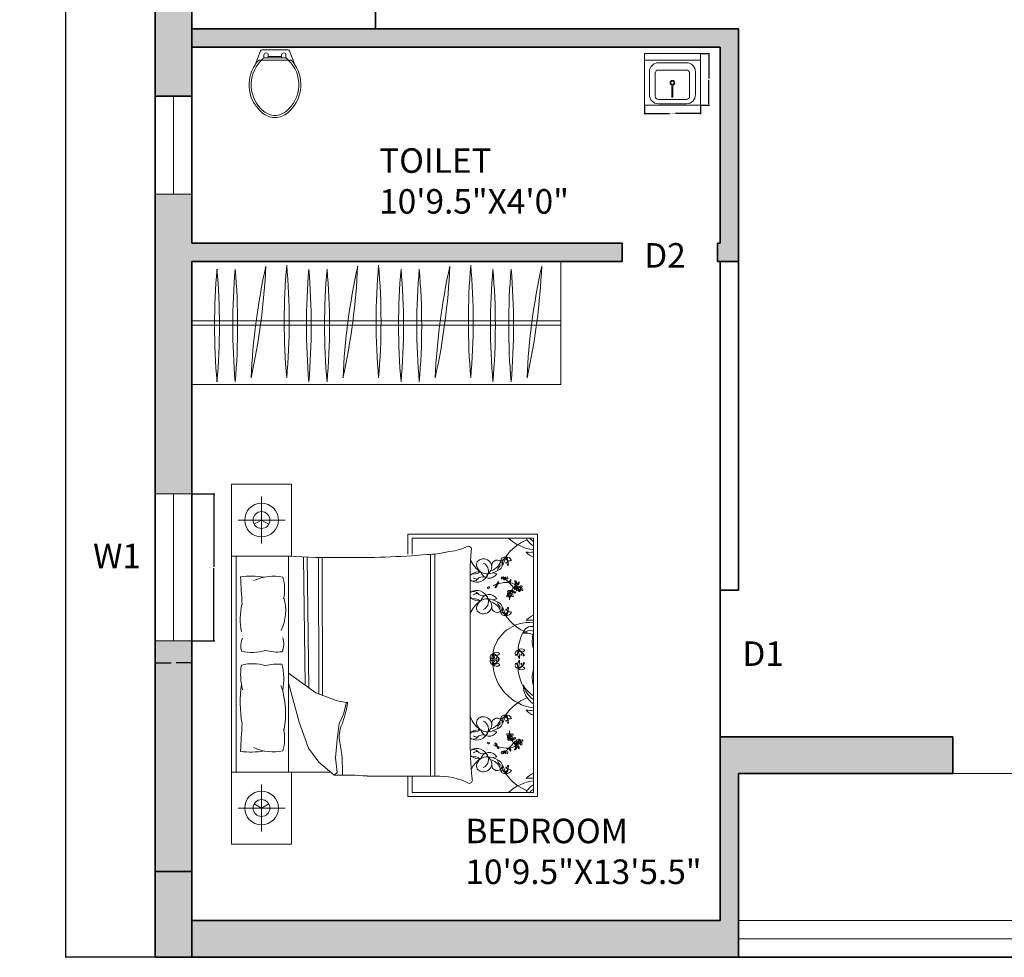
# Model space of a CAD drawing. Units: inches. Extents: x -9 to 505, y -680 to 48.
# Tile 1 of 17: x -6 to 235, y -680 to -450. Entities that reach past the tile are written whole.
import ezdxf

# ---------------------------------------------------------------- set-up
doc = ezdxf.new("R2010")
doc.units = ezdxf.units.IN
doc.header["$MEASUREMENT"] = 0
for name, color, linetype, lineweight in [('A-ANNO-DIMS', 2, 'Continuous', 18), ('A-ANNO-TEXT', 7, 'Continuous', 18), ('A-AREA-IDEN', 7, 'Continuous', 18), ('A-FLOR-CASE', 8, 'Continuous', 18), ('A-FLOR-FIXT', 9, 'Continuous', 18), ('A-FLOR-HRAL', 4, 'Continuous', 18), ('A-FURN', 8, 'Continuous', 18), ('A-GLAZ', 4, 'Continuous', 18), ('A-WALL', 7, 'Continuous', 35), ('A-WALL-PATT', 251, 'Continuous', 13), ('S-CONC', 7, 'Continuous', 35), ('S-CONC-PATT', 18, 'Continuous', 13), ('WC-Detail_dwgmodels.com', 251, 'Continuous', 13), ('WC-Outline_dwgmodels.com', 250, 'Continuous', 18)]:
    doc.layers.add(name, color=color, linetype=linetype, lineweight=lineweight)
doc.styles.get("Standard").update_dxf_attribs({"font": 'arial.ttf'})
doc.dimstyles.get("Standard").update_dxf_attribs({"dimtxt": 0.18, "dimasz": 0.18, "dimexe": 0.18, "dimexo": 0.0625, "dimgap": 0.09, "dimtad": 0, "dimtih": 1, "dimtoh": 1, "dimdec": 0, "dimzin": 0, "dimdsep": 46, "dimlunit": 3, "dimtxsty": 'Standard', "dimcen": 0.09, "dimadec": 0, "dimazin": 0, "dimtfac": 1, "dimtdec": 0, "dimtofl": 0, "dimtmove": 0, "dimatfit": 3, "dimfxl": 1, "dimtolj": 1, "dimtzin": 0, "dimarcsym": 0})

# ---------------------------------------------------------------- blocks, each defined once
blk = doc.blocks.new('*D3')
at = {"layer": 'A-ANNO-DIMS', "color": 0, "lineweight": -2, "transparency": 16777216}
for p, q in [((27.2, 11.5), (5.16, 11.5)), ((5.34, 11.32), (5.34, -330.86)), ((5.34, -679.32), (5.34, -337.14)), ((27.2, -679.5), (5.16, -679.5))]:
    blk.add_line(p, q, dxfattribs=at)
at = {"layer": 'A-ANNO-DIMS', "color": 0, "transparency": 16777216}
for points in [[(5.31, 11.32), (5.37, 11.32), (5.34, 11.5)], [(5.31, -679.32), (5.37, -679.32), (5.34, -679.5)]]:
    blk.add_solid(points, dxfattribs=at)
at = {"layer": 'Defpoints', "color": 0, "transparency": 16777216}
for p in [(27.26, 11.5), (5.34, -679.5), (27.26, -679.5)]:
    blk.add_point(p, dxfattribs=at)
at = {"layer": 'A-ANNO-DIMS', "color": 0, "transparency": 16777216, "insert": (5.34, -334), "char_height": 6, "attachment_point": 5}
blk.add_mtext('\\A1;57\'-7"', dxfattribs=at)
blk = doc.blocks.new('М14 600х655')
for p, q in [((-655, 600), (-655, 0)), ((-655, 600), (-655, 0)), ((-655, 0), (-655, 600)), ((0, 600), (-655, 600)), ((0, 0), (0, 600)), ((0, 525), (-655, 525)), ((-165, 494), (-490, 494)), ((-596, 388), (-596, 121)), ((-528, 370), (-528, 103)), ((-165, 408), (-490, 408)), ((-127, 103), (-127, 370)), ((-59, 121), (-59, 388)), ((-334, 87), (-334, 220)), ((-321, 87), (-321, 220)), ((-655, 0), (-655, 0)), ((-655, 0), (-655, 0)), ((-655, 0), (0, 0)), ((-655, 0), (0, 0)), ((-490, 65), (-165, 65)), ((-490, 15), (-165, 15))]:
    blk.add_line(p, q)
for radius in [27.6, 19.3]:
    blk.add_circle((-327, 259), radius)
for centre, radius, start, end in [((-490, 388), 106, 90, 180), ((-165, 388), 106, 0, 90), ((-490, 370), 38.2, 90, 180), ((-165, 370), 38.2, 0, 90), ((-490, 121), 106, 180, 270), ((-165, 121), 106, 270, 0), ((-490, 103), 38.2, 180, 270), ((-165, 103), 38.2, 270, 0)]:
    blk.add_arc(centre, radius, start, end)
blk = doc.blocks.new('WIN-36')
for p, q in [((0, 36), (0, 0)), ((9, 36), (0, 36)), ((4.5, 36), (4.5, 2.23)), ((9, 0), (9, 36)), ((0, 0), (9, 0)), ((4.5, 2.23), (4.5, 0))]:
    blk.add_line(p, q)
blk = doc.blocks.new('WIN-24')
for p, q in [((0, 24), (0, 0)), ((9, 24), (0, 24)), ((4.5, 24), (4.5, 2.23)), ((9, 0), (9, 24)), ((0, 0), (9, 0)), ((4.5, 2.23), (4.5, 0))]:
    blk.add_line(p, q)
blk = doc.blocks.new('*D16')
at = {"layer": 'A-ANNO-DIMS', "color": 0, "lineweight": -2, "transparency": 16777216}
for p, q in [((36.33, -565.96), (41.84, -565.96)), ((41.66, -566.14), (41.66, -583.78)), ((41.66, -601.78), (41.66, -584.14)), ((36.33, -601.96), (41.84, -601.96))]:
    blk.add_line(p, q, dxfattribs=at)
at = {"layer": 'A-ANNO-DIMS', "color": 0, "transparency": 16777216}
for points in [[(41.63, -566.14), (41.69, -566.14), (41.66, -565.96)], [(41.63, -601.78), (41.69, -601.78), (41.66, -601.96)]]:
    blk.add_solid(points, dxfattribs=at)
at = {"layer": 'Defpoints', "color": 0, "transparency": 16777216}
for p in [(36.26, -565.96), (41.66, -565.96), (36.26, -601.96)]:
    blk.add_point(p, dxfattribs=at)
at = {"layer": 'A-ANNO-DIMS', "color": 0, "transparency": 16777216, "insert": (41.66, -583.96), "char_height": 0.18, "attachment_point": 5}
blk.add_mtext('\\A1;WINDOW 3\'-0" TYP.', dxfattribs=at)
blk = doc.blocks.new('*D17')
at = {"layer": 'A-ANNO-DIMS', "color": 0, "lineweight": -2, "transparency": 16777216}
for p, q in [((27.26, -602.02), (27.26, -607.54)), ((36.26, -602.02), (36.26, -607.54)), ((27.44, -607.36), (31.12, -607.36)), ((36.08, -607.36), (32.4, -607.36))]:
    blk.add_line(p, q, dxfattribs=at)
at = {"layer": 'A-ANNO-DIMS', "color": 0, "transparency": 16777216}
for points in [[(27.44, -607.33), (27.44, -607.39), (27.26, -607.36)], [(36.08, -607.33), (36.08, -607.39), (36.26, -607.36)]]:
    blk.add_solid(points, dxfattribs=at)
at = {"layer": 'Defpoints', "color": 0, "transparency": 16777216}
for p in [(27.26, -601.96), (36.26, -601.96), (36.26, -607.36)]:
    blk.add_point(p, dxfattribs=at)
at = {"layer": 'A-ANNO-DIMS', "color": 0, "transparency": 16777216, "insert": (31.76, -607.36), "char_height": 0.18, "attachment_point": 5}
blk.add_mtext('\\A1;0\'-9" TYP.', dxfattribs=at)
blk = doc.blocks.new('*D30')
at = {"layer": 'A-ANNO-DIMS', "color": 0, "lineweight": -2, "transparency": 16777216}
for p, q in [((147.17, -470.73), (147.17, -472.91)), ((147.35, -472.73), (153.31, -472.73)), ((160.75, -472.73), (154.79, -472.73)), ((160.93, -470.73), (160.93, -472.91))]:
    blk.add_line(p, q, dxfattribs=at)
at = {"layer": 'A-ANNO-DIMS', "color": 0, "transparency": 16777216}
for points in [[(147.35, -472.7), (147.35, -472.76), (147.17, -472.73)], [(160.75, -472.7), (160.75, -472.76), (160.93, -472.73)]]:
    blk.add_solid(points, dxfattribs=at)
at = {"layer": 'Defpoints', "color": 0, "transparency": 16777216}
for p in [(147.17, -470.66), (160.93, -470.66), (160.93, -472.73)]:
    blk.add_point(p, dxfattribs=at)
at = {"layer": 'A-ANNO-DIMS', "color": 0, "transparency": 16777216, "insert": (154.05, -472.73), "char_height": 0.18, "attachment_point": 5}
blk.add_mtext('\\A1;BASIN 1\'-2"', dxfattribs=at)
blk = doc.blocks.new('*D31')
at = {"layer": 'A-ANNO-DIMS', "color": 0, "lineweight": -2, "transparency": 16777216}
for p, q in [((160.99, -458.06), (163.18, -458.06)), ((163, -458.24), (163, -464.18)), ((163, -470.48), (163, -464.54)), ((160.99, -470.66), (163.18, -470.66))]:
    blk.add_line(p, q, dxfattribs=at)
at = {"layer": 'A-ANNO-DIMS', "color": 0, "transparency": 16777216}
for points in [[(162.97, -458.24), (163.03, -458.24), (163, -458.06)], [(162.97, -470.48), (163.03, -470.48), (163, -470.66)]]:
    blk.add_solid(points, dxfattribs=at)
at = {"layer": 'Defpoints', "color": 0, "transparency": 16777216}
for p in [(160.93, -458.06), (163, -458.06), (160.93, -470.66)]:
    blk.add_point(p, dxfattribs=at)
at = {"layer": 'A-ANNO-DIMS', "color": 0, "transparency": 16777216, "insert": (163, -464.36), "char_height": 0.18, "attachment_point": 5}
blk.add_mtext('\\A1;1\'-0 1/2"', dxfattribs=at)

msp = doc.modelspace()

# ---------------------------------------------------------------- hatches: boundary and pattern name
at = {"layer": 'A-WALL-PATT'}
h = msp.add_hatch(color=256, dxfattribs=at)
h.dxf.hatch_style = 1
h.paths.add_polyline_path([(101.64, 11.5), (48.26, 11.5), (48.26, 2.5), (72.26, 2.5), (72.26, -21.25), (81.26, -21.25), (81.26, 2.5), (101.64, 2.5)])
h.paths.add_polyline_path([(36.26, 2.5), (27.26, 2.5), (27.26, -6.92), (36.26, -6.92)])
h.paths.add_polyline_path([(81.26, -57.25), (72.26, -57.25), (72.26, -75.5), (81.26, -75.5)])
h.paths.add_polyline_path([(162.76, 11.5), (137.64, 11.5), (137.64, 2.5), (162.76, 2.5)])
h.paths.add_polyline_path([(179.26, 2.5), (174.76, 2.5), (174.76, -75.5), (179.26, -75.5), (179.26, -54.5), (229.51, -54.5), (229.51, -45.5), (179.26, -45.5)])
h.paths.add_polyline_path([(382.26, -45.5), (332.26, -45.5), (332.26, 2.5), (327.76, 2.5), (327.76, -45.5), (277.51, -45.5), (277.51, -54.5), (327.76, -54.5), (327.76, -111.5), (332.26, -111.5), (332.26, -54.5), (382.26, -54.5)])
h.paths.add_polyline_path([(332.26, -128), (327.76, -128), (327.76, -207), (332.26, -207)])
h.paths.add_polyline_path([(124.76, -111.5), (36.26, -111.5), (36.26, -116), (120.26, -116), (120.26, -168.5), (179.26, -168.5), (179.26, -164), (124.76, -164)])
h.paths.add_polyline_path([(96.26, -164), (36.26, -164), (36.26, -152), (27.26, -152), (27.26, -208.88), (36.26, -208.88), (36.26, -168.5), (96.26, -168.5)])
h.paths.add_polyline_path([(36.26, -244.88), (27.26, -244.88), (27.26, -287), (36.26, -287)])
h.paths.add_polyline_path([(179.26, -204.5), (174.76, -204.5), (174.76, -287), (179.26, -287)])
h.paths.add_polyline_path([(257.26, -296), (248.26, -296), (248.26, -446), (269.26, -446), (269.26, -437), (257.26, -437)])
h.paths.add_polyline_path([(90.26, -296), (81.26, -296), (81.26, -348.67), (90.26, -348.67)])
h.paths.add_polyline_path([(90.26, -384.67), (81.26, -384.67), (81.26, -416), (90.26, -416)])
h.paths.add_polyline_path([(170.26, -452), (36.26, -452), (36.26, -456.5), (165.76, -456.5), (165.76, -504.5), (165.13, -504.5), (165.13, -509), (170.26, -509)])
h.paths.add_polyline_path([(141.76, -504.5), (36.26, -504.5), (36.26, -492.5), (27.26, -492.5), (27.26, -565.96), (36.26, -565.96), (36.26, -509), (141.76, -509)])
h.paths.add_polyline_path([(36.26, -601.96), (27.26, -601.96), (27.26, -658.5), (36.26, -658.5)])
h.paths.add_polyline_path([(170.26, -670.5), (170.26, -634.5), (222.76, -634.5), (222.76, -625.5), (165.76, -625.5), (165.76, -670.5), (36.26, -670.5), (36.26, -679.5), (170.26, -679.5)])
h.paths.add_polyline_path([(332.26, -616.5), (433.89, -616.5), (433.89, -612), (332.26, -612), (332.26, -610.56), (327.76, -610.56), (327.76, -625.5), (270.76, -625.5), (270.76, -634.5), (327.76, -634.5), (327.76, -658.5), (332.26, -658.5)])
h.paths.add_polyline_path([(459.76, -670.5), (336.76, -670.5), (336.76, -679.5), (459.76, -679.5)])
h.paths.add_polyline_path([(468.76, -545.74), (459.76, -545.74), (459.76, -612), (457.89, -612), (457.89, -616.5), (459.76, -616.5), (459.76, -658.5), (468.76, -658.5)])
h.paths.add_polyline_path([(332.26, -446), (327.76, -446), (327.76, -574.56), (332.26, -574.56)])
h.paths.add_polyline_path([(327.76, -437), (305.26, -437), (305.26, -446), (327.76, -446)])
h.paths.add_polyline_path([(459.76, -437), (348.76, -437), (348.76, -446), (459.76, -446)])
h.paths.add_polyline_path([(468.76, -458), (459.76, -458), (459.76, -509.74), (468.76, -509.74)])
h.paths.add_polyline_path([(468.76, -365), (459.76, -365), (459.76, -437), (468.76, -437)])
h.paths.add_polyline_path([(468.76, -299.6), (459.76, -299.6), (459.76, -344), (468.76, -344)])
h.paths.add_polyline_path([(468.76, -184.74), (459.76, -184.74), (459.76, -231), (401.26, -231), (401.26, -235.5), (459.76, -235.5), (459.76, -275.6), (468.76, -275.6)])
h.paths.add_polyline_path([(390.76, -356), (342.76, -356), (342.76, -365), (390.76, -365)])
h.paths.add_polyline_path([(459.76, -356), (405.76, -356), (405.76, -365), (459.76, -365)])
h.paths.add_polyline_path([(405.76, -296), (396.76, -296), (396.76, -356), (405.76, -356)])
h.paths.add_polyline_path([(336.76, -296), (327.76, -296), (327.76, -356), (336.76, -356)])
h.paths.add_polyline_path([(468.76, -9.5), (459.76, -9.5), (459.76, -45.5), (418.26, -45.5), (418.26, -54.5), (468.76, -54.5)])
h.paths.add_polyline_path([(468.76, -54.5), (459.76, -54.5), (459.76, -111.5), (468.76, -111.5)])
h.paths.add_polyline_path([(468.76, -128), (459.76, -128), (459.76, -148.74), (468.76, -148.74)])
at = {"layer": 'S-CONC-PATT'}
h = msp.add_hatch(color=256, dxfattribs=at)
h.dxf.hatch_style = 1
h.paths.add_polyline_path([(36.26, -447.5), (27.26, -447.5), (27.26, -468.5), (36.26, -468.5), (36.26, -456.5), (36.26, -452)])
h = msp.add_hatch(color=256, dxfattribs=at)
h.dxf.hatch_style = 1
h.paths.add_polyline_path([(336.76, -658.5), (327.76, -658.5), (327.76, -679.5), (336.76, -679.5), (336.76, -670.5)])
h.paths.add_polyline_path([(468.76, -658.5), (459.76, -658.5), (459.76, -679.5), (468.76, -679.5)])
h.paths.add_polyline_path([(36.26, -658.5), (27.26, -658.5), (27.26, -679.5), (36.26, -679.5)])

# ---------------------------------------------------------------- linework, layer by layer
at = {"layer": 'A-FLOR-CASE'}
for p, q in [((126.66, -509), (36.26, -509)), ((36.26, -509), (36.26, -539.13)), ((126.66, -509), (126.66, -539.13)), ((126.66, -523.56), (36.26, -523.56)), ((126.66, -524.57), (36.26, -524.57)), ((126.66, -539.13), (36.26, -539.13))]:
    msp.add_line(p, q, dxfattribs=at)
for centre, start, end in [((200.34, -524.67), 175.0028, 184.9972), ((-115.55, -524.67), 355.0028, 4.9972), ((204.8, -524.67), 175.0028, 184.9972), ((-111.08, -524.67), 355.0028, 4.9972), ((-104.03, -503.22), 347.508, 357.5023), ((209.16, -544.42), 167.508, 177.5023), ((217.43, -523.7), 175.0028, 184.9972), ((-98.45, -523.7), 355.0028, 4.9972), ((222.86, -524.67), 175.0028, 184.9972), ((-93.03, -524.67), 355.0028, 4.9972), ((227.32, -524.67), 175.0028, 184.9972), ((-88.56, -524.67), 355.0028, 4.9972), ((-81.51, -503.22), 347.508, 357.5023), ((231.68, -544.42), 167.508, 177.5023), ((239.95, -523.7), 175.0028, 184.9972), ((-75.93, -523.7), 355.0028, 4.9972), ((245.46, -524.67), 175.0028, 184.9972), ((-70.42, -524.67), 355.0028, 4.9972), ((249.93, -524.67), 175.0028, 184.9972), ((-65.96, -524.67), 355.0028, 4.9972), ((254.28, -544.42), 167.508, 177.5023), ((-58.9, -503.22), 347.508, 357.5023), ((262.56, -523.7), 175.0028, 184.9972), ((-53.33, -523.7), 355.0028, 4.9972), ((267.98, -524.67), 175.0028, 184.9972), ((-47.9, -524.67), 355.0028, 4.9972), ((272.45, -524.67), 175.0028, 184.9972), ((-43.43, -524.67), 355.0028, 4.9972), ((276.8, -544.42), 167.508, 177.5023), ((-36.38, -503.22), 347.508, 357.5023)]:
    msp.add_arc(centre, 158.54, start, end, dxfattribs=at)
at = {"layer": 'A-FLOR-HRAL'}
for p, q in [((170.26, -670.5), (170.26, -679.5)), ((327.76, -670.5), (170.26, -670.5)), ((170.26, -670.5), (327.76, -670.5)), ((170.26, -675), (327.76, -675)), ((170.26, -679.5), (327.76, -679.5))]:
    msp.add_line(p, q, dxfattribs=at)
at = {"layer": 'A-FURN'}
for p, q in [((45.97, -651.75), (45.97, -563.54)), ((53.32, -578.12), (53.32, -566.59)), ((59.09, -572.36), (47.56, -572.36)), ((89.21, -580.69), (89.21, -575.8)), ((89.21, -575.8), (120.99, -575.8)), ((90.23, -576.82), (90.23, -580.71)), ((119.97, -576.82), (90.23, -576.82)), ((119.97, -639.08), (119.97, -576.82)), ((120.99, -575.8), (120.99, -640.1)), ((47.1, -581.18), (47.1, -634.11)), ((59.91, -634.11), (59.91, -581.18)), ((63.58, -581.42), (64.02, -612.82)), ((64.48, -581.45), (64.93, -613.48)), ((67.26, -581.5), (67.39, -614.99)), ((68.16, -581.49), (68.3, -615.34)), ((94.71, -580.78), (94.71, -635.12)), ((95.81, -580.69), (95.81, -635.12)), ((111.02, -585.51), (110.03, -585.32)), ((104.48, -589.73), (104.48, -625.55)), ((111.02, -591.67), (110.03, -591.87)), ((59.91, -609.87), (66.64, -614.71)), ((62.53, -621.85), (59.91, -612.23)), ((66.64, -614.71), (71.82, -616.67)), ((71.82, -616.67), (74.14, -617.03)), ((74.14, -617.03), (73.42, -619.89)), ((73.42, -619.89), (72.35, -622.21)), ((64.85, -628.28), (62.53, -621.85)), ((72.35, -622.21), (71.82, -626.14)), ((111.02, -624.22), (110.03, -624.03)), ((71.82, -626.14), (71.46, -630.61)), ((67.35, -631.68), (64.85, -628.28)), ((71.1, -634.89), (67.35, -631.68)), ((71.46, -630.61), (71.82, -634.18)), ((111.02, -630.39), (110.03, -630.58)), ((45.97, -634.11), (70.18, -634.11)), ((71.82, -634.18), (71.1, -634.89)), ((53.32, -637.16), (53.32, -648.69)), ((89.21, -640.1), (89.21, -635.11)), ((90.23, -635.12), (90.23, -639.08)), ((90.23, -639.08), (119.97, -639.08)), ((120.99, -640.1), (89.21, -640.1)), ((59.09, -642.93), (47.56, -642.93))]:
    msp.add_line(p, q, dxfattribs=at)
for points in [[(45.97, -581.18), (60.67, -581.18), (60.67, -563.54), (45.97, -563.54)], [(53.32, -572.36), (51.54, -573.39)], [(53.32, -572.36), (55.1, -573.39)], [(60.67, -634.11), (60.67, -651.75), (45.97, -651.75)], [(53.32, -642.93), (51.54, -641.9)], [(53.32, -642.93), (55.1, -641.9)]]:
    msp.add_lwpolyline(points, dxfattribs=at)
for points in [[(94.02, -580.8, 0.056112), (98.87, -580.16, 0.095341), (103.55, -578.92)], [(48.17, -586.25, -0.074897), (53.93, -586.35, 0.472817)], [(54.25, -604.29, -0.14099), (48.38, -604.46, -0.235245)], [(54.25, -608.06, 0.14099), (48.38, -607.88, 0.235245)], [(48.17, -629.04, 0.074897), (53.93, -628.93, -0.472817)], [(79.18, -635.08, 0.001242), (95.92, -635.12, -0.127202), (104.26, -636.89)]]:
    msp.add_lwpolyline(points, format="xyb", dxfattribs=at)
for centre, radius in [((53.32, -572.36), 4.12), ((53.32, -572.36), 2.06), ((116.59, -589.14), 0.225), ((114.22, -590.61), 0.225), ((114.22, -625.29), 0.225), ((116.59, -626.76), 0.225), ((53.32, -642.93), 4.12), ((53.32, -642.93), 2.06)]:
    msp.add_circle(centre, radius, dxfattribs=at)
for centre, radius, start, end in [((121.52, -568.24), 11.52, 228.1144, 262.255), ((123.06, -574.02), 5.61, 209.8884, 236.5383), ((124.11, -572), 6.99, 223.5186, 233.6964), ((104, -579.59), 0.804, 336.5219, 123.8264), ((122.66, -587.95), 11.52, 111.4092, 145.6135), ((70.69, -423.05), 158.5, 266.1, 270.9282), ((76.45, -374.79), 206.76, 269.1145, 274.8735), ((190.27, -587.03), 85.84, 175.2402, 181.8035), ((112.92, -582.37), 0.955, 76.272, 177.0484), ((111.47, -580.42), 1.97, 284.7031, 328.6173), ((114.22, -582.92), 1.82, 125.7657, 194.5347), ((105.28, -579.7), 8.06, 332.8176, 347.4827), ((113.42, -582.69), 1.28, 20.9613, 102.2885), ((114.11, -581.41), 0.962, 181.7131, 301.5367), ((110.96, -583.36), 2.91, 2.0648, 41.1598), ((112.71, -582.28), 0.942, 316.2238, 62.3173), ((121.76, -577.16), 4.68, 221.0454, 247.4453), ((119.25, -564.33), 15.94, 266.3481, 272.5919), ((110.69, -579.48), 6.68, 203.6453, 236.3329), ((107.49, -583.37), 1.49, 88.9462, 185.5144), ((108.59, -582.91), 2.65, 193.079, 274.7067), ((107.7, -583.98), 2.11, 7.1143, 95.0551), ((106.9, -584.81), 2.05, 338.5779, 68.4181), ((107.23, -583.61), 2.56, 305.9599, 357.6409), ((108.18, -580.87), 4.16, 288.2955, 328.7386), ((111.09, -583.49), 1.32, 19.1312, 189.736), ((110.7, -583.17), 1.65, 285.6955, 4.031), ((112.89, -584.96), 1.76, 128.4175, 173.8338), ((112.53, -583.22), 0.811, 126.7319, 206.0245), ((113.26, -582.83), 0.0751, 20.2667, 316.2271), ((113.73, -583.26), 0.143, 168.5166, 2.0648), ((113.65, -583.25), 0.0695, 52.0591, 168.5166), ((-791.3, -634.87), 840.88, 2.85022, 3.31479), ((56.24, -597.48), 11.37, 78.2417, 114.8684), ((47.14, -589.39), 11.82, 348.9631, 14.8961), ((105.45, -586.45), 1.06, 127.675, 162.5814), ((105.13, -581.93), 3.65, 259.249, 301.1782), ((106.08, -584.76), 2.81, 240.8249, 340.7178), ((106.72, -588.43), 3.4, 85.2696, 124.215), ((106.59, -584.33), 2.54, 240.0851, 262.564), ((107.58, -588.08), 1.81, 74.8529, 138.4347), ((109.12, -584.42), 2.19, 196.8663, 330.0915), ((108.2, -585.81), 0.547, 254.8529, 12.6959), ((106.72, -588.43), 3.4, 53.6555, 57.2989), ((108.52, -580.83), 4.73, 273.4924, 303.7117), ((112.27, -586.63), 0.174, 125.0752, 284.7644), ((112.54, -586.56), 0.375, 127.3642, 168.4363), ((112.24, -586.26), 0.54, 277.4968, 341.2737), ((112.67, -586.51), 0.215, 88.1325, 178.8919), ((113.1, -586.74), 0.464, 136.3462, 189.6513), ((112.88, -586.25), 0.225, 183.2768, 356.7232), ((113.59, -586.65), 0.735, 164.2829, 186.9148), ((112.72, -586.66), 0.368, 312.3208, 40.2111), ((113.5, -586.24), 0.522, 201.6382, 274.947), ((112.81, -586.96), 0.682, 42.3896, 66.5724), ((113.3, -586.56), 0.371, 10.9597, 52.2379), ((113.53, -586.59), 0.172, 274.947, 37.5263), ((105.45, -586.45), 1.06, 196.6343, 225.5483), ((105.24, -586), 1.32, 246.1646, 318.4347), ((108.93, -588.83), 0.276, 169.5864, 349.5616), ((109.03, -588.85), 0.17, 349.5616, 167.2949), ((113.47, -594.96), 7.31, 110.1059, 116.9968), ((111.02, -588.94), 0.463, 129.5056, 182.6421), ((109.69, -587.87), 1.39, 308.4388, 328.836), ((109.45, -586.73), 2.49, 296.5064, 305.3102), ((109.43, -588.01), 1.42, 336.3901, 344.4871), ((110.97, -588.37), 0.18, 83.9457, 185.6216), ((110.25, -588.21), 0.739, 328.836, 0.8141), ((110.63, -588.42), 0.423, 306.5232, 32.4668), ((111.14, -588.09), 0.18, 112.5583, 214.2343), ((111.02, -587.77), 0.423, 265.7131, 351.6568), ((110.65, -587.54), 0.739, 297.3659, 329.344), ((110.09, -586.9), 1.42, 313.6929, 321.7899), ((111.66, -587.87), 0.463, 115.5379, 168.6744), ((110.09, -587.21), 1.39, 329.344, 349.7412), ((113.47, -594.96), 7.31, 86.1723, 106.4158), ((108.97, -587.53), 2.49, 352.8698, 1.6736), ((112.84, -586.79), 0.194, 189.6513, 312.3208), ((119.69, -581.56), 8.38, 217.9541, 226.8459), ((114.11, -587.57), 0.18, 112.5583, 214.2343), ((113.99, -587.25), 0.423, 265.7131, 351.6568), ((113.62, -587.01), 0.739, 297.3659, 329.344), ((113.66, -591.32), 3.66, 60.7959, 85.244), ((105.86, -596.59), 12.05, 37.8256, 47.7588), ((113.06, -586.38), 1.42, 313.6929, 321.7899), ((114.63, -587.35), 0.463, 115.5379, 168.6744), ((113.06, -586.68), 1.39, 329.344, 349.7412), ((111.94, -587), 2.49, 352.8698, 1.6736), ((118.52, -591.7), 4.39, 130.182, 149.456), ((115.44, -587.5), 0.251, 33.0979, 123.1364), ((109.91, -591.04), 6.56, 31.1156, 34.8118), ((115.08, -587.93), 0.679, 2.3172, 70.5201), ((116.1, -589.19), 0.724, 139.3812, 199.9959), ((114.75, -588.67), 1.02, 310.9365, 22.7695), ((115.64, -588.1), 0.196, 135.7354, 318.1297), ((115.31, -587.78), 0.26, 315.7354, 31.1156), ((115.09, -588.33), 0.603, 319.3812, 5.5456), ((115.78, -588.1), 0.196, 68.2452, 250.6395), ((115.33, -587.86), 0.585, 352.6008, 57.1845), ((117.42, -591.78), 3.91, 111.7087, 116.2181), ((113.66, -591.32), 3.66, 47.5083, 55.9967), ((115.89, -587.72), 0.585, 252.8042, 349.6943), ((115.33, -588.77), 0.622, 331.1838, 51.6792), ((115.95, -587.68), 0.26, 248.2452, 323.6254), ((115.72, -587.52), 0.679, 291.7087, 3.0299), ((116.19, -588.85), 0.22, 138.2946, 276.2474), ((116.28, -588.89), 0.306, 358.5719, 143.8954), ((110.88, -583.94), 6.56, 323.6254, 327.3216), ((116.45, -588.65), 0.309, 208.8493, 269.9355), ((116.19, -588.72), 0.353, 274.2123, 318.1587), ((116.26, -587.69), 0.251, 325.6077, 55.6462), ((117.27, -589.08), 0.708, 121.9501, 165.2442), ((116.78, -588.8), 0.149, 262.868, 7.094), ((116.76, -588.68), 0.443, 278.5614, 22.5914), ((117.01, -588.66), 0.223, 44.3732, 121.9501), ((48.01, -594.49), 11.23, 333.8761, 16.1746), ((105.45, -590.73), 1.06, 134.4517, 156.7144), ((105.45, -590.73), 1.06, 203.2856, 232.325), ((106.08, -592.43), 2.81, 19.2822, 119.1751), ((105.24, -591.18), 1.32, 41.5653, 113.8354), ((106.59, -592.85), 2.54, 97.436, 119.9149), ((107.58, -589.11), 1.81, 221.5653, 285.1471), ((109.12, -592.77), 2.19, 29.9085, 163.1337), ((108.2, -591.38), 0.547, 347.3041, 105.1471), ((113.6, -590.98), 0.174, 125.0752, 284.7644), ((113.87, -590.92), 0.375, 93.635, 168.4363), ((113.89, -588.89), 1.02, 253.6301, 325.4631), ((114.17, -590.31), 0.724, 82.0748, 142.6895), ((114.09, -589.31), 0.744, 228.342, 274.9894), ((113.82, -590.32), 0.22, 138.2946, 276.2474), ((113.58, -590.62), 0.54, 277.4968, 341.2737), ((113.91, -590.36), 0.306, 358.5719, 143.8954), ((114.01, -590.87), 0.215, 88.1325, 178.8919), ((114.09, -590.12), 0.309, 208.8493, 269.9355), ((113.82, -590.19), 0.353, 274.2123, 318.1587), ((114.44, -591.1), 0.464, 136.3462, 189.6513), ((114.17, -591.14), 0.194, 189.6513, 312.3208), ((118.52, -591.7), 4.39, 175.2415, 182.8929), ((114.11, -589.43), 0.622, 273.8774, 357.1501), ((114.92, -591.01), 0.735, 164.2829, 186.9148), ((114.9, -590.55), 0.708, 121.9501, 165.2442), ((114.36, -588.99), 0.603, 262.0748, 308.2393), ((114.05, -591.01), 0.368, 312.3208, 40.2111), ((114.83, -590.6), 0.522, 201.6382, 274.947), ((114.41, -590.27), 0.149, 262.868, 7.094), ((114.14, -591.31), 0.682, 42.3896, 66.5724), ((114.39, -590.15), 0.443, 278.5614, 22.5914), ((114.64, -590.91), 0.371, 10.9597, 118.7804), ((118.52, -591.7), 4.39, 156.1523, 156.9499), ((114.64, -590.13), 0.223, 44.3732, 121.9501), ((115.33, -589.61), 0.622, 181.4625, 249.4747), ((115.22, -589.12), 0.603, 215.1128, 261.2773), ((115.7, -589.15), 1.02, 197.889, 269.722), ((114.86, -590.95), 0.172, 274.947, 37.5263), ((115.38, -589.5), 0.744, 248.3627, 295.0101), ((115.02, -590.43), 0.724, 20.6625, 81.2773), ((115.22, -588.73), 0.744, 285.6484, 332.2957), ((115.97, -589.51), 0.174, 125.0752, 284.7644), ((116.24, -589.45), 0.375, 93.635, 168.4363), ((115.95, -589.15), 0.54, 277.4968, 341.2737), ((116.38, -589.4), 0.215, 88.1325, 178.8919), ((116.81, -589.63), 0.464, 136.3462, 189.6513), ((116.54, -589.67), 0.194, 189.6513, 312.3208), ((117.29, -589.54), 0.735, 164.2829, 186.9148), ((116.42, -589.54), 0.368, 312.3208, 40.2111), ((117.2, -589.13), 0.522, 201.6382, 274.947), ((116.51, -589.84), 0.682, 42.3896, 66.5724), ((117, -589.44), 0.371, 10.9597, 118.7804), ((117.23, -589.48), 0.172, 274.947, 37.5263), ((63.6, -596.71), 15.51, 166.3427, 191.1841), ((105.13, -595.26), 3.65, 58.8218, 100.2867), ((110.69, -597.71), 6.68, 123.6671, 158.5059), ((106.72, -588.76), 3.4, 235.785, 274.7304), ((108.59, -594.28), 2.65, 85.2933, 166.921), ((107.49, -593.82), 1.49, 174.4856, 271.0538), ((107.7, -593.21), 2.11, 264.9449, 352.8857), ((106.9, -592.38), 2.05, 291.5819, 21.4221), ((106.72, -588.76), 3.4, 302.7011, 306.3445), ((107.23, -593.57), 2.56, 2.3591, 54.0401), ((108.52, -596.36), 4.73, 56.2883, 86.5076), ((108.18, -596.32), 4.16, 31.2614, 71.7045), ((111.09, -593.69), 1.32, 170.264, 340.8688), ((112.89, -592.23), 1.76, 186.1662, 231.5825), ((110.7, -594.01), 1.65, 355.969, 74.3045), ((112.53, -593.97), 0.811, 153.9755, 233.2681), ((114.22, -594.26), 1.82, 165.4653, 234.2343), ((105.28, -597.49), 8.06, 12.5173, 27.1824), ((113.73, -593.92), 0.143, 357.9352, 191.4834), ((112.92, -594.81), 0.955, 182.9516, 283.728), ((111.47, -596.77), 1.97, 31.3827, 75.2969), ((110.96, -593.82), 2.91, 318.8402, 357.9352), ((112.71, -594.91), 0.942, 297.6827, 43.7762), ((114.11, -595.77), 0.962, 58.4633, 178.2869), ((113.42, -594.49), 1.28, 257.7115, 339.0387), ((122.66, -589.24), 11.52, 214.3865, 248.5908), ((113.3, -594.34), 0.125, 43.7762, 339.7183), ((113.65, -593.94), 0.0695, 191.4834, 307.9409), ((121.76, -600.02), 4.68, 112.5547, 138.9546), ((118.86, -606.38), 8.91, 82.8636, 171.8197), ((119.48, -600.49), 2.07, 76.3898, 169.0739), ((119.25, -612.85), 15.94, 87.4081, 93.6519), ((127.69, -605.12), 11.52, 152.5854, 175.5377), ((119.2, -602.05), 2.61, 72.8609, 131.9049), ((118.04, -605.22), 5.16, 68.117, 96.6195), ((126.02, -601.9), 6.33, 162.9798, 196.4569), ((52.57, -603.25), 4.36, 153.3437, 196.1026), ((54.09, -602.66), 4.68, 335.0183, 18.5407), ((57.2, -593.89), 10.81, 254.1707, 275.9871), ((110.3, -606.02), 0.955, 106.1963, 206.9726), ((108.07, -605.06), 1.97, 314.6273, 358.5415), ((111.69, -605.86), 1.82, 155.6899, 224.4589), ((111.69, -607.1), 1.82, 135.5411, 204.3101), ((110.89, -606.05), 1.28, 50.8855, 132.2127), ((110.85, -604.6), 0.962, 211.6373, 331.4609), ((110.07, -606.05), 0.942, 346.148, 92.2415), ((109.09, -607.86), 2.91, 31.989, 71.0841), ((102.35, -607.52), 8.06, 2.7418, 17.407), ((102.35, -605.44), 8.06, 342.593, 357.2582), ((116.47, -605.14), 0.955, 106.1963, 206.9726), ((114.24, -604.17), 1.97, 314.6273, 358.5415), ((117.86, -604.97), 1.82, 155.6899, 224.4589), ((117.06, -605.17), 1.28, 50.8855, 132.2127), ((117.02, -603.72), 0.962, 211.6373, 331.4609), ((115.26, -606.98), 2.91, 31.989, 71.0841), ((108.52, -606.64), 8.06, 2.7418, 17.407), ((116.24, -605.17), 0.942, 346.148, 92.2415), ((116.99, -605.37), 0.0751, 50.1909, 346.0209), ((117.61, -605.51), 0.143, 198.4408, 31.989), ((117.54, -605.54), 0.0695, 81.9833, 198.4408), ((129.29, -604.41), 9.37, 174.3643, 175.6213), ((135.7, -609.34), 16.74, 160.0972, 160.2783), ((63.92, -610.2), 15.72, 171.5249, 193.96), ((57.2, -618.45), 10.81, 84.0129, 105.8293), ((43.21, -611.37), 15.56, 349.8617, 13.6238), ((110.3, -606.94), 0.955, 153.0274, 253.8037), ((108.07, -607.9), 1.97, 1.4585, 45.3727), ((109.09, -605.1), 2.91, 288.9159, 328.011), ((110.07, -606.91), 0.942, 267.7585, 13.852), ((110.85, -608.36), 0.962, 28.5391, 148.3627), ((110.89, -606.91), 1.28, 227.7873, 309.1145), ((121.52, -606.96), 11.52, 184.4623, 262.255), ((110.82, -606.26), 0.0751, 50.1909, 346.0209), ((110.87, -606.72), 0.125, 13.852, 309.9245), ((111.44, -606.4), 0.143, 198.4408, 31.989), ((111.37, -606.42), 0.0695, 81.9833, 198.4408), ((111.44, -606.56), 0.143, 328.011, 161.5592), ((111.37, -606.54), 0.0695, 161.5592, 278.0167), ((116.47, -607.82), 0.955, 153.0274, 253.8037), ((114.24, -608.78), 1.97, 1.4585, 45.3727), ((117.86, -607.98), 1.82, 135.5411, 204.3101), ((108.52, -606.32), 8.06, 342.593, 357.2582), ((115.26, -605.98), 2.91, 288.9159, 328.011), ((116.24, -607.79), 0.942, 267.7585, 13.852), ((117.02, -609.24), 0.962, 28.5391, 148.3627), ((117.04, -607.6), 0.125, 13.852, 309.9245), ((117.61, -607.45), 0.143, 328.011, 161.5592), ((117.54, -607.42), 0.0695, 161.5592, 278.0167), ((117.06, -607.79), 1.28, 227.7873, 309.1145), ((127.69, -607.84), 11.52, 184.4623, 207.4146), ((126.02, -611.06), 6.33, 163.5431, 197.0202), ((129.29, -608.55), 9.37, 184.3787, 185.6357), ((135.7, -603.62), 16.74, 199.7217, 199.9028), ((80.09, -616.95), 31.99, 172.2196, 189.497), ((38.73, -619.67), 20.5, 348.0397, 19.2615), ((123.06, -612.73), 5.61, 181.272, 236.5383), ((126.07, -607.04), 10.4, 214.0123, 234.053), ((124.11, -610.72), 6.99, 197.8504, 233.6964), ((40.81, -610.9), 34.21, 340.1194, 349.3383), ((74.21, -617.23), 0.213, 358.8623, 109.7536), ((122.66, -626.66), 11.52, 111.4092, 145.6135), ((112.92, -621.09), 0.955, 76.272, 177.0484), ((111.47, -619.13), 1.97, 284.7031, 328.6173), ((114.22, -621.64), 1.82, 125.7657, 194.5347), ((105.28, -618.41), 8.06, 332.8176, 347.4827), ((113.42, -621.41), 1.28, 20.9613, 102.2885), ((112.71, -620.99), 0.942, 316.2238, 62.3173), ((110.96, -622.08), 2.91, 2.0648, 41.1598), ((114.11, -620.13), 0.962, 181.7131, 301.5367), ((119.25, -603.05), 15.94, 266.3481, 272.5919), ((121.76, -615.88), 4.68, 221.0454, 247.4453), ((-791.3, -580.42), 840.88, 356.68521, 357.14978), ((79.55, -625.43), 7.18, 156.2616, 191.3392), ((110.69, -618.19), 6.68, 201.4941, 236.3329), ((107.49, -622.08), 1.49, 88.9462, 185.5144), ((108.59, -621.62), 2.65, 193.079, 274.7067), ((107.7, -622.69), 2.11, 7.1143, 95.0551), ((106.9, -623.52), 2.05, 338.5779, 68.4181), ((107.23, -622.33), 2.56, 305.9599, 357.6409), ((108.18, -619.58), 4.16, 288.2955, 328.7386), ((111.09, -622.21), 1.32, 19.1312, 189.736), ((110.7, -621.89), 1.65, 285.6955, 4.031), ((112.89, -623.67), 1.76, 128.4175, 173.8338), ((112.53, -621.93), 0.811, 126.7319, 206.0245), ((113.26, -621.54), 0.0751, 20.2667, 316.2271), ((113.73, -621.98), 0.143, 168.5166, 2.0648), ((113.65, -621.96), 0.0695, 52.0591, 168.5166), ((47.14, -625.89), 11.82, 345.1039, 11.0369), ((105.13, -620.64), 3.65, 259.7133, 301.1782), ((105.45, -625.17), 1.06, 127.675, 156.7144), ((106.08, -623.47), 2.81, 240.8249, 340.7178), ((106.72, -627.14), 3.4, 85.2696, 124.215), ((107.58, -626.79), 1.81, 74.8529, 138.4347), ((109.12, -623.13), 2.19, 196.8663, 330.0915), ((108.2, -624.52), 0.547, 254.8529, 12.6959), ((106.72, -627.14), 3.4, 53.6555, 57.2989), ((108.52, -619.54), 4.73, 273.4924, 303.7117), ((113.6, -624.92), 0.174, 75.2356, 234.9248), ((113.87, -624.98), 0.375, 191.5637, 266.365), ((113.58, -625.28), 0.54, 18.7263, 82.5032), ((114.01, -625.03), 0.215, 181.1081, 271.8675), ((114.44, -624.8), 0.464, 170.3487, 223.6538), ((114.17, -624.76), 0.194, 47.6792, 170.3487), ((118.52, -624.2), 4.39, 177.1071, 184.7585), ((114.92, -624.89), 0.735, 173.0852, 195.7171), ((114.05, -624.89), 0.368, 319.7889, 47.6792), ((114.83, -625.3), 0.522, 85.053, 158.3618), ((114.14, -624.59), 0.682, 293.4276, 317.6104), ((114.64, -624.99), 0.371, 241.2196, 349.0403), ((114.86, -624.95), 0.172, 322.4737, 85.053), ((39.87, -633.39), 33.29, 357.4519, 11.3392), ((196.3, -626.6), 91.83, 179.3433, 185.6887), ((105.45, -625.17), 1.06, 203.229, 225.5483), ((105.24, -624.72), 1.32, 246.1646, 318.4347), ((106.59, -623.05), 2.54, 240.0851, 262.564), ((108.93, -627.07), 0.276, 10.4384, 190.4136), ((109.03, -627.05), 0.17, 192.7051, 10.4384), ((113.47, -620.94), 7.31, 243.0032, 249.8941), ((109.69, -628.03), 1.39, 31.164, 51.5612), ((111.02, -626.96), 0.463, 177.3579, 230.4944), ((109.45, -629.17), 2.49, 54.6898, 63.4936), ((109.43, -627.89), 1.42, 15.5129, 23.6099), ((110.97, -627.52), 0.18, 174.3784, 276.0543), ((110.25, -627.69), 0.739, 359.1859, 31.164), ((110.63, -627.48), 0.423, 327.5332, 53.4768), ((113.82, -625.58), 0.22, 83.7526, 221.7054), ((114.09, -626.59), 0.744, 85.0106, 131.658), ((113.89, -627.01), 1.02, 34.5369, 106.3699), ((114.17, -625.59), 0.724, 217.3105, 277.9252), ((113.91, -625.54), 0.306, 216.1046, 1.4281), ((114.09, -625.78), 0.309, 90.0645, 151.1507), ((113.82, -625.71), 0.353, 41.8413, 85.7877), ((105.86, -619.31), 12.05, 312.2412, 322.1744), ((114.11, -626.47), 0.622, 2.8499, 86.1226), ((114.9, -625.35), 0.708, 194.7558, 238.0499), ((114.36, -626.91), 0.603, 51.7607, 97.9252), ((114.41, -625.63), 0.149, 352.906, 97.132), ((114.39, -625.75), 0.443, 337.4086, 81.4386), ((118.52, -624.2), 4.39, 203.0501, 203.8477), ((114.64, -625.77), 0.223, 238.0499, 315.6268), ((115.33, -626.29), 0.622, 110.5253, 178.5375), ((115.7, -626.75), 1.02, 90.278, 162.111), ((115.22, -626.78), 0.603, 98.7227, 144.8872), ((118.52, -624.2), 4.39, 210.544, 229.818), ((115.38, -626.4), 0.744, 64.9899, 111.6373), ((115.02, -625.47), 0.724, 278.7227, 339.3375), ((116.1, -626.7), 0.724, 160.0041, 220.6188), ((114.75, -627.23), 1.02, 337.2305, 49.0635), ((115.22, -627.17), 0.744, 27.7043, 74.3516), ((115.64, -627.8), 0.196, 41.8703, 224.2646), ((115.09, -627.57), 0.603, 354.4544, 40.6188), ((113.66, -624.58), 3.66, 304.0033, 312.4917), ((115.33, -627.13), 0.622, 308.3208, 28.8162), ((115.89, -628.17), 0.585, 10.3057, 107.1958), ((115.97, -626.39), 0.174, 75.2356, 234.9248), ((116.24, -626.45), 0.375, 191.5637, 266.365), ((116.19, -627.04), 0.22, 83.7526, 221.7054), ((115.95, -626.75), 0.54, 18.7263, 82.5032), ((116.28, -627.01), 0.306, 216.1046, 1.4281), ((116.38, -626.5), 0.215, 181.1081, 271.8675), ((116.45, -627.25), 0.309, 90.0645, 151.1507), ((116.19, -627.18), 0.353, 41.8413, 85.7877), ((116.81, -626.27), 0.464, 170.3487, 223.6538), ((116.54, -626.23), 0.194, 47.6792, 170.3487), ((117.29, -626.36), 0.735, 173.0852, 195.7171), ((117.27, -626.82), 0.708, 194.7558, 238.0499), ((116.42, -626.36), 0.368, 319.7889, 47.6792), ((117.2, -626.77), 0.522, 85.053, 158.3618), ((116.78, -627.1), 0.149, 352.906, 97.132), ((116.51, -626.06), 0.682, 293.4276, 317.6104), ((117, -626.46), 0.371, 241.2196, 349.0403), ((116.76, -627.22), 0.443, 337.4086, 81.4386), ((117.01, -627.23), 0.223, 238.0499, 315.6268), ((117.23, -626.42), 0.172, 322.4737, 85.053), ((56.24, -617.8), 11.37, 245.1316, 281.7583), ((105.45, -629.45), 1.06, 134.4517, 153.558), ((105.45, -629.45), 1.06, 210.0293, 232.325), ((106.08, -631.14), 2.81, 19.2822, 119.1751), ((105.24, -629.9), 1.32, 41.5653, 113.8354), ((106.59, -631.57), 2.54, 97.436, 119.9149), ((107.58, -627.82), 1.81, 221.5653, 285.1471), ((109.12, -631.48), 2.19, 29.9085, 163.1337), ((108.2, -630.09), 0.547, 347.3041, 105.1471), ((111.14, -627.8), 0.18, 145.7657, 247.4417), ((111.02, -628.13), 0.423, 8.3432, 94.2869), ((110.65, -628.36), 0.739, 30.656, 62.6341), ((110.09, -629), 1.42, 38.2101, 46.3071), ((111.66, -628.03), 0.463, 191.3256, 244.4621), ((110.09, -628.69), 1.39, 10.2588, 30.656), ((113.47, -620.94), 7.31, 253.5842, 273.8277), ((108.97, -628.37), 2.49, 358.3264, 7.1302), ((112.27, -629.27), 0.174, 75.2356, 234.9248), ((112.54, -629.34), 0.375, 191.5637, 232.6358), ((112.24, -629.64), 0.54, 18.7263, 82.5032), ((112.67, -629.39), 0.215, 181.1081, 271.8675), ((113.1, -629.16), 0.464, 170.3487, 223.6538), ((112.84, -629.11), 0.194, 47.6792, 170.3487), ((112.88, -629.65), 0.225, 3.2768, 176.7232), ((113.59, -629.25), 0.735, 173.0852, 195.7171), ((112.72, -629.24), 0.368, 319.7889, 47.6792), ((113.5, -629.66), 0.522, 85.053, 158.3618), ((119.69, -634.34), 8.38, 133.1541, 142.0459), ((112.81, -628.94), 0.682, 293.4276, 317.6104), ((113.3, -629.34), 0.371, 307.7621, 349.0403), ((113.53, -629.31), 0.172, 322.4737, 85.053), ((114.11, -628.33), 0.18, 145.7657, 247.4417), ((113.66, -624.58), 3.66, 274.756, 299.2041), ((113.99, -628.65), 0.423, 8.3432, 94.2869), ((113.62, -628.89), 0.739, 30.656, 62.6341), ((113.06, -629.52), 1.42, 38.2101, 46.3071), ((114.63, -628.55), 0.463, 191.3256, 244.4621), ((113.06, -629.22), 1.39, 10.2588, 30.656), ((111.94, -628.9), 2.49, 358.3264, 7.1302), ((115.08, -627.97), 0.679, 289.4799, 357.6828), ((109.91, -624.86), 6.56, 325.1882, 328.8844), ((115.44, -628.4), 0.251, 236.8636, 326.9021), ((115.31, -628.12), 0.26, 328.8844, 44.2646), ((115.78, -627.8), 0.196, 109.3605, 291.7548), ((115.33, -628.04), 0.585, 302.8155, 7.3992), ((117.42, -624.12), 3.91, 243.7819, 248.2913), ((115.95, -628.22), 0.26, 36.3746, 111.7548), ((115.72, -628.38), 0.679, 356.9701, 68.2913), ((110.88, -631.96), 6.56, 32.6784, 36.3746), ((116.26, -628.21), 0.251, 304.3538, 34.3923), ((105.13, -633.97), 3.65, 58.8218, 99.1554), ((110.69, -636.42), 6.68, 123.6671, 153.2997), ((106.72, -627.47), 3.4, 235.785, 274.7304), ((108.59, -632.99), 2.65, 85.2933, 166.921), ((107.49, -632.53), 1.49, 174.4856, 271.0538), ((107.7, -631.92), 2.11, 264.9449, 352.8857), ((106.9, -631.09), 2.05, 291.5819, 21.4221), ((106.72, -627.47), 3.4, 302.7011, 306.3445), ((107.23, -632.29), 2.56, 2.3591, 54.0401), ((108.52, -635.07), 4.73, 56.2883, 86.5076), ((108.18, -635.03), 4.16, 31.2614, 71.7045), ((111.09, -632.41), 1.32, 170.264, 340.8688), ((110.7, -632.72), 1.65, 355.969, 74.3045), ((112.89, -630.94), 1.76, 186.1662, 231.5825), ((112.53, -632.68), 0.811, 153.9755, 233.2681), ((111.47, -635.48), 1.97, 31.3827, 75.2969), ((112.92, -633.53), 0.955, 182.9516, 283.728), ((114.22, -632.98), 1.82, 165.4653, 234.2343), ((105.28, -636.2), 8.06, 12.5173, 27.1824), ((110.96, -632.54), 2.91, 318.8402, 357.9352), ((112.71, -633.62), 0.942, 297.6827, 43.7762), ((114.11, -634.48), 0.962, 58.4633, 178.2869), ((113.42, -633.21), 1.28, 257.7115, 339.0387), ((122.66, -627.95), 11.52, 214.3865, 248.5908), ((113.3, -633.06), 0.125, 43.7762, 339.7183), ((113.73, -632.64), 0.143, 357.9352, 191.4834), ((113.65, -632.65), 0.0695, 191.4834, 307.9409), ((121.76, -638.74), 4.68, 112.5547, 138.9546), ((73.3, -715.77), 80.91, 85.8294, 91.553), ((104.2, -636.08), 0.814, 273.98, 27.3412), ((121.52, -647.66), 11.52, 97.745, 131.8856), ((123.06, -641.88), 5.61, 123.4617, 150.1116), ((119.25, -651.56), 15.94, 87.4081, 93.6519), ((124.11, -643.9), 6.99, 126.3036, 136.4814)]:
    msp.add_arc(centre, radius, start, end, dxfattribs=at)
at = {"layer": 'A-GLAZ'}
msp.add_line((222.76, -634.5), (270.76, -634.5), dxfattribs=at)
at = {"layer": 'A-WALL'}
for p, q in [((27.26, 11.5), (27.26, -679.5)), ((36.26, -296), (36.26, -452)), ((81.26, -416), (81.26, -452)), ((36.26, -452), (170.26, -452)), ((170.26, -452), (170.26, -589.5)), ((36.26, -456.5), (165.76, -456.5)), ((36.26, -456.5), (36.26, -504.5)), ((165.76, -456.5), (165.76, -504.5)), ((36.26, -504.5), (141.76, -504.5)), ((141.76, -504.5), (141.76, -509)), ((165.13, -504.5), (165.13, -509)), ((165.13, -504.5), (165.76, -504.5)), ((36.26, -509), (141.76, -509)), ((36.26, -509), (36.26, -679.5)), ((165.13, -509), (170.26, -509)), ((165.76, -509), (165.76, -670.5)), ((170.26, -589.5), (165.76, -589.5)), ((165.76, -625.5), (222.76, -625.5)), ((222.76, -634.5), (222.76, -625.5)), ((170.26, -634.5), (222.76, -634.5)), ((170.26, -634.5), (170.26, -679.5)), ((36.26, -670.5), (165.76, -670.5)), ((27.26, -679.5), (468.76, -679.5))]:
    msp.add_line(p, q, dxfattribs=at)
at = {"layer": 'S-CONC'}
for p, q in [((36.26, -452), (36.26, -456.5)), ((36.26, -468.5), (27.26, -468.5)), ((36.26, -658.5), (27.26, -658.5))]:
    msp.add_line(p, q, dxfattribs=at)
at = {"layer": 'WC-Detail_dwgmodels.com'}
for p, q in [((52.65, -459.63), (53.34, -459.63)), ((59.88, -459.63), (60.58, -459.63))]:
    msp.add_line(p, q, dxfattribs=at)
for points in [[(53.92, -459.13), (53.92, -458.43, -1), (54.98, -458.43), (54.98, -458.79)], [(59.31, -459.13), (59.31, -458.43, 1), (58.25, -458.43), (58.25, -458.79)], [(52.65, -459.63, 0.040937), (51.75, -460.77, 0.163732)], [(53.92, -459.13, 0.022712), (53.34, -459.63, 0.162618)], [(56.61, -459.13), (53.92, -459.13, 0.022712)], [(56.61, -459.13), (59.31, -459.13, -0.476108)], [(59.31, -459.13, -0.022712), (59.88, -459.63, -0.162618)], [(60.58, -459.63, -0.040937), (61.48, -460.77, -0.163732)]]:
    msp.add_lwpolyline(points, format="xyb", dxfattribs=at)
for points in [[(58.25, -458.79), (54.98, -458.79)], [(54.98, -458.79), (54.98, -459.13)], [(58.25, -458.79), (58.25, -459.13)]]:
    msp.add_lwpolyline(points, dxfattribs=at)
at = {"layer": 'WC-Outline_dwgmodels.com'}
for p in [(53.34, -459.63), (59.88, -459.63)]:
    msp.add_line(p, (56.61, -459.63), dxfattribs=at)
for points in [[(56.61, -457.11), (53.44, -457.11, 0.31031), (53.05, -457.38), (51.75, -460.77, 0.209071)], [(56.61, -457.11), (59.79, -457.11, -0.31031), (60.18, -457.38), (61.48, -460.77, -0.209071)], [(51.75, -460.77, 0.383919), (53.49, -472.54, 0.163732), (56.61, -473.74, 0.359733)], [(53.01, -459.97, 0.431639), (53.81, -472.15, 0.162618), (56.61, -473.24, 0.470877)], [(53.34, -459.63, 0.014165), (53.01, -459.97, 0.162618)], [(59.88, -459.63, -0.448546), (59.42, -472.15, -0.162618), (56.61, -473.24, -0.470877)], [(61.48, -460.77, -0.383919), (59.74, -472.54, -0.163732), (56.61, -473.74, -0.359733)]]:
    msp.add_lwpolyline(points, format="xyb", dxfattribs=at)

# ---------------------------------------------------------------- block references
at = {"layer": 'A-FLOR-FIXT', "xscale": 0.0210106819292851, "yscale": 0.0210106819292851, "zscale": 0.0210106819292851}
msp.add_blockref('М14 600х655', (160.93, -470.66), dxfattribs=at)
at = {"layer": 'A-GLAZ'}
for name, p in [('WIN-24', (27.26, -492.5)), ('WIN-36', (27.26, -601.96))]:
    msp.add_blockref(name, p, dxfattribs=at)

# ---------------------------------------------------------------- texts
at = {"layer": 'A-ANNO-TEXT', "insert": (147.15, -504.5), "char_height": 6, "attachment_point": 1}
msp.add_mtext_dynamic_manual_height_columns('D2', width=0.3266, gutter_width=1, heights=[0], dxfattribs=at)
at = {"layer": 'A-ANNO-TEXT', "char_height": 6, "attachment_point": 1}
for s, insert in [('W1', (12.02, -578.15)), ('D1', (171.21, -602.09))]:
    msp.add_mtext(s, dxfattribs=dict(at, insert=insert))
at = {"layer": 'A-AREA-IDEN', "char_height": 6, "attachment_point": 1}
for s, insert in [('TOILET\\P10\'9.5"X4\'0"', (82.16, -481.27)), ('BEDROOM\\P10\'9.5"X13\'5.5"', (103.31, -645.54))]:
    msp.add_mtext(s, dxfattribs=dict(at, insert=insert))

# ---------------------------------------------------------------- dimensions: what is measured, and where the dimension line sits
at = {"layer": 'A-ANNO-DIMS'}
for base, p1, p2, override, picture, middle in [((5.34, -679.5), (27.26, 11.5), (27.26, -679.5), {"dimtxt": 6, "dimclrd": 0, "dimclre": 0, "dimclrt": 0}, '*D3', (5.34, -334)), ((163, -458.06), (160.93, -470.66), (160.93, -458.06), {"dimdec": 1, "dimlfac": 1, "dimrnd": 0, "dimzin": 1, "dimdsep": 46, "dimlunit": 4, "dimfrac": 2}, '*D31', (163, -464.36))]:
    dim = msp.add_linear_dim(base=base, p1=p1, p2=p2, angle=90, dimstyle='Standard', override=override, dxfattribs=at)
    dim.commit()
    dim.dimension.update_dxf_attribs({"geometry": picture, "text_midpoint": middle})
for base, p1, p2, text, picture, middle in [((160.93, -472.73), (147.17, -470.66), (160.93, -470.66), 'BASIN <>', '*D30', (154.05, -472.73)), ((36.26, -607.36), (27.26, -601.96), (36.26, -601.96), '<> TYP.', '*D17', (31.76, -607.36))]:
    dim = msp.add_linear_dim(base=base, p1=p1, p2=p2, text=text, dimstyle='Standard', override={"dimdec": 1, "dimlfac": 1, "dimrnd": 0, "dimzin": 1, "dimdsep": 46, "dimlunit": 4, "dimfrac": 2}, dxfattribs=at)
    dim.commit()
    dim.dimension.update_dxf_attribs({"geometry": picture, "text_midpoint": middle})
dim = msp.add_linear_dim(base=(41.66, -565.96), p1=(36.26, -601.96), p2=(36.26, -565.96), angle=90, text='WINDOW <> TYP.', dimstyle='Standard', override={"dimdec": 1, "dimlfac": 1, "dimrnd": 0, "dimzin": 1, "dimdsep": 46, "dimlunit": 4, "dimfrac": 2}, dxfattribs=at)
dim.commit()
dim.dimension.update_dxf_attribs({"geometry": '*D16', "text_midpoint": (41.66, -583.96)})

doc.saveas('drawing.dxf')
